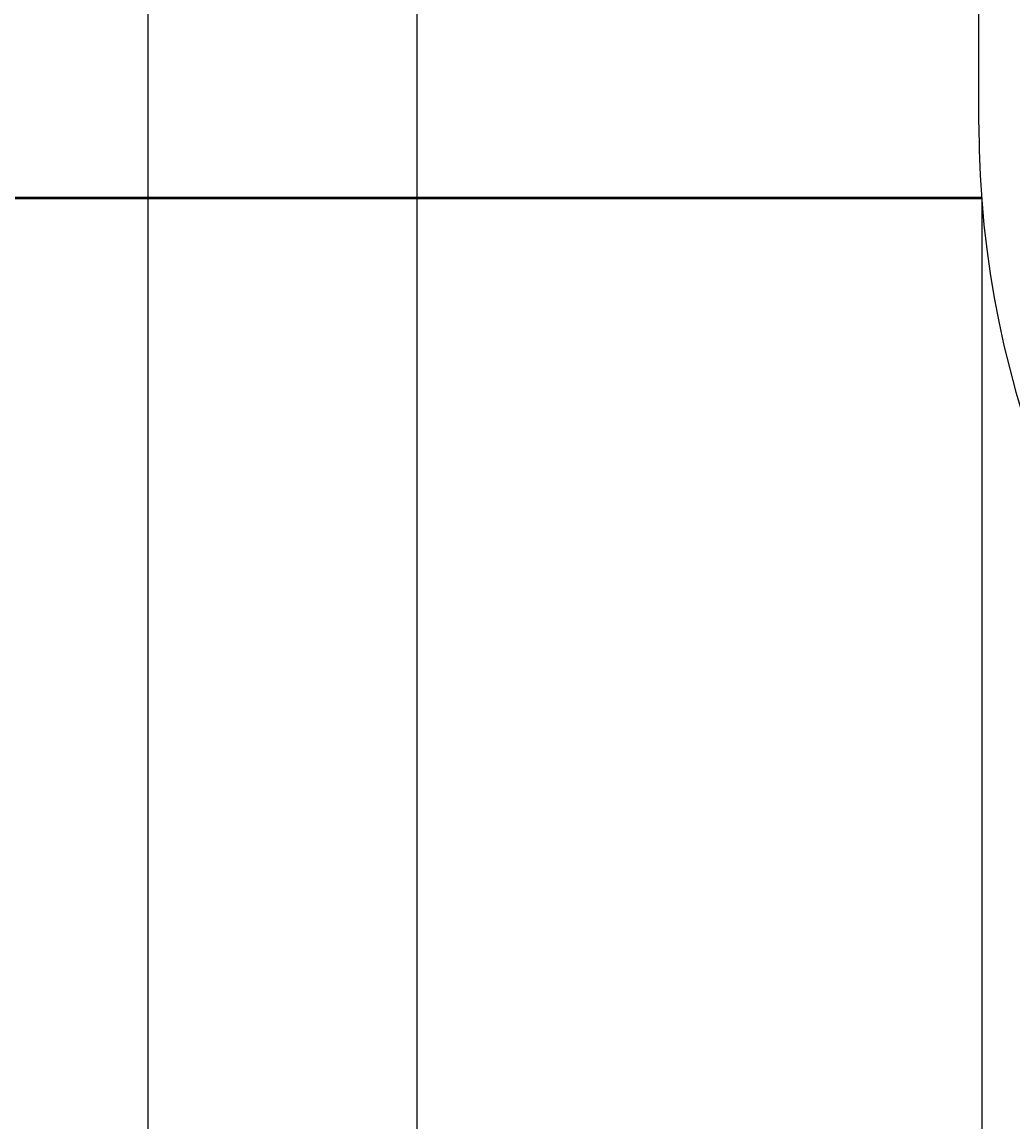
# Model space of a CAD drawing. Units: inches. Extents: x 37 to 824, y -700 to 234.
# Tile 34 of 77: x 211 to 251, y -206 to -161. Entities that reach past the tile are written whole.
import ezdxf

# ---------------------------------------------------------------- set-up
doc = ezdxf.new("R2010")
doc.units = ezdxf.units.IN
doc.header["$MEASUREMENT"] = 0
for name, color, linetype, lineweight in [('A-ANNO-DIMS', 2, 'Continuous', 18), ('A-DOOR', 4, 'Continuous', 25), ('A-WALL', 2, 'Continuous', 50)]:
    doc.layers.add(name, color=color, linetype=linetype, lineweight=lineweight)
doc.styles.get("Standard").update_dxf_attribs({"font": 'arial.ttf'})
doc.dimstyles.get("Standard").update_dxf_attribs({"dimtxt": 0.18, "dimasz": 0.18, "dimexe": 0.18, "dimexo": 0.0625, "dimgap": 0.09, "dimtad": 0, "dimtih": 1, "dimtoh": 1, "dimdec": 1, "dimzin": 0, "dimdsep": 46, "dimlunit": 4, "dimtxsty": 'Standard', "dimcen": 0.09, "dimadec": 0, "dimazin": 0, "dimtfac": 1, "dimtdec": 1, "dimtofl": 0, "dimtmove": 0, "dimatfit": 3, "dimfxl": 1, "dimtolj": 1, "dimtzin": 0, "dimarcsym": 0})

# ---------------------------------------------------------------- blocks, each defined once
blk = doc.blocks.new('*U2')
blk.add_line((-40, 0), (-40, 6))
blk.add_arc((0, 0), 40, 180, 270)
blk = doc.blocks.new('*D77')
at = {"layer": 'A-ANNO-DIMS', "color": 0, "lineweight": -2, "ltscale": 0.5, "transparency": 16777216}
for p, q in [((227.077, 45.5), (227.077, -400.406)), ((290.077, 15.028), (290.077, -400.406)), ((227.257, -400.226), (258.248, -400.226)), ((289.897, -400.226), (258.906, -400.226))]:
    blk.add_line(p, q, dxfattribs=at)
at = {"layer": 'A-ANNO-DIMS', "color": 0, "ltscale": 0.5, "transparency": 16777216}
for points in [[(227.257, -400.196), (227.257, -400.256), (227.077, -400.226)], [(289.897, -400.196), (289.897, -400.256), (290.077, -400.226)]]:
    blk.add_solid(points, dxfattribs=at)
at = {"layer": 'Defpoints', "color": 0, "ltscale": 0.5, "transparency": 16777216}
for p in [(227.077, 45.563), (290.077, 15.09), (290.077, -400.226)]:
    blk.add_point(p, dxfattribs=at)
at = {"layer": 'A-ANNO-DIMS', "color": 0, "ltscale": 0.5, "transparency": 16777216, "insert": (258.577, -400.226), "char_height": 0.18, "attachment_point": 5}
blk.add_mtext('\\A1;5\'-3"', dxfattribs=at)
blk = doc.blocks.new('*D80')
at = {"layer": 'A-ANNO-DIMS', "color": 0, "lineweight": -2, "ltscale": 0.5, "transparency": 16777216}
for p, q in [((170.077, -167.972), (170.077, -400.406)), ((250.19, -167.972), (250.19, -400.406)), ((170.257, -400.226), (209.804, -400.226)), ((250.01, -400.226), (210.463, -400.226))]:
    blk.add_line(p, q, dxfattribs=at)
at = {"layer": 'A-ANNO-DIMS', "color": 0, "ltscale": 0.5, "transparency": 16777216}
for points in [[(170.257, -400.196), (170.257, -400.256), (170.077, -400.226)], [(250.01, -400.196), (250.01, -400.256), (250.19, -400.226)]]:
    blk.add_solid(points, dxfattribs=at)
at = {"layer": 'Defpoints', "color": 0, "ltscale": 0.5, "transparency": 16777216}
for p in [(170.077, -167.91), (250.19, -167.91), (250.19, -400.226)]:
    blk.add_point(p, dxfattribs=at)
at = {"layer": 'A-ANNO-DIMS', "color": 0, "ltscale": 0.5, "transparency": 16777216, "insert": (210.133, -400.226), "char_height": 0.18, "attachment_point": 5}
blk.add_mtext('\\A1;6\'-8"', dxfattribs=at)
blk = doc.blocks.new('*D81')
at = {"layer": 'A-ANNO-DIMS', "color": 0, "lineweight": -2, "ltscale": 0.5, "transparency": 16777216}
for p, q in [((290.077, -164.972), (290.077, -400.406)), ((250.19, -167.972), (250.19, -400.406)), ((250.37, -400.226), (269.804, -400.226)), ((289.897, -400.226), (270.463, -400.226))]:
    blk.add_line(p, q, dxfattribs=at)
at = {"layer": 'A-ANNO-DIMS', "color": 0, "ltscale": 0.5, "transparency": 16777216}
for points in [[(250.37, -400.196), (250.37, -400.256), (250.19, -400.226)], [(289.897, -400.196), (289.897, -400.256), (290.077, -400.226)]]:
    blk.add_solid(points, dxfattribs=at)
at = {"layer": 'Defpoints', "color": 0, "ltscale": 0.5, "transparency": 16777216}
for p in [(290.077, -164.91), (250.19, -167.91), (290.077, -400.226)]:
    blk.add_point(p, dxfattribs=at)
at = {"layer": 'A-ANNO-DIMS', "color": 0, "ltscale": 0.5, "transparency": 16777216, "insert": (270.133, -400.226), "char_height": 0.18, "attachment_point": 5}
blk.add_mtext('\\A1;3\'-4"', dxfattribs=at)
blk = doc.blocks.new('*D86')
at = {"layer": 'A-ANNO-DIMS', "color": 0, "lineweight": -2, "ltscale": 0.5, "transparency": 16777216}
for p, q in [((206.077, -356.847), (206.077, 234.17)), ((206.257, 233.99), (210.678, 233.99)), ((215.897, 233.99), (211.476, 233.99)), ((216.077, -356.847), (216.077, 234.17))]:
    blk.add_line(p, q, dxfattribs=at)
at = {"layer": 'A-ANNO-DIMS', "color": 0, "ltscale": 0.5, "transparency": 16777216}
for points in [[(206.257, 234.02), (206.257, 233.96), (206.077, 233.99)], [(215.897, 234.02), (215.897, 233.96), (216.077, 233.99)]]:
    blk.add_solid(points, dxfattribs=at)
at = {"layer": 'Defpoints', "color": 0, "ltscale": 0.5, "transparency": 16777216}
for p in [(216.077, 233.99), (206.077, -356.91), (216.077, -356.91)]:
    blk.add_point(p, dxfattribs=at)
at = {"layer": 'A-ANNO-DIMS', "color": 0, "ltscale": 0.5, "transparency": 16777216, "insert": (211.077, 233.99), "char_height": 0.18, "attachment_point": 5}
blk.add_mtext('\\A1;0\'-10"', dxfattribs=at)
blk = doc.blocks.new('*D87')
at = {"layer": 'A-ANNO-DIMS', "color": 0, "lineweight": -2, "ltscale": 0.5, "transparency": 16777216}
for p, q in [((216.077, -356.847), (216.077, 234.17)), ((216.257, 233.99), (255.747, 233.99)), ((295.897, 233.99), (256.407, 233.99)), ((296.077, -356.847), (296.077, 234.17))]:
    blk.add_line(p, q, dxfattribs=at)
at = {"layer": 'A-ANNO-DIMS', "color": 0, "ltscale": 0.5, "transparency": 16777216}
for points in [[(216.257, 234.02), (216.257, 233.96), (216.077, 233.99)], [(295.897, 234.02), (295.897, 233.96), (296.077, 233.99)]]:
    blk.add_solid(points, dxfattribs=at)
at = {"layer": 'Defpoints', "color": 0, "ltscale": 0.5, "transparency": 16777216}
for p in [(296.077, 233.99), (216.077, -356.91), (296.077, -356.91)]:
    blk.add_point(p, dxfattribs=at)
at = {"layer": 'A-ANNO-DIMS', "color": 0, "ltscale": 0.5, "transparency": 16777216, "insert": (256.077, 233.99), "char_height": 0.18, "attachment_point": 5}
blk.add_mtext('\\A1;6\'-8"', dxfattribs=at)

msp = doc.modelspace()

# ---------------------------------------------------------------- linework, layer by layer
at = {"layer": 'A-WALL'}
msp.add_line((250.19, -167.91), (170.077, -167.91), dxfattribs=at)

# ---------------------------------------------------------------- block references
at = {"layer": 'A-DOOR'}
msp.add_blockref('*U2', (290.077, -164.91), dxfattribs=at)

# ---------------------------------------------------------------- dimensions: what is measured, and where the dimension line sits
at = {"layer": 'A-ANNO-DIMS', "ltscale": 0.5}
for base, p1, p2, picture, middle in [((216.077, 233.99), (206.077, -356.91), (216.077, -356.91), '*D86', (211.077, 233.99)), ((296.077, 233.99), (216.077, -356.91), (296.077, -356.91), '*D87', (256.077, 233.99)), ((290.077, -400.226), (227.077, 45.563), (290.077, 15.09), '*D77', (258.577, -400.226)), ((290.077, -400.226), (250.19, -167.91), (290.077, -164.91), '*D81', (270.133, -400.226)), ((250.19, -400.226), (170.077, -167.91), (250.19, -167.91), '*D80', (210.133, -400.226))]:
    dim = msp.add_linear_dim(base=base, p1=p1, p2=p2, dimstyle='Standard', override={"dimdec": 1, "dimlfac": 1, "dimrnd": 0, "dimzin": 1, "dimdsep": 46, "dimlunit": 4, "dimfrac": 2}, dxfattribs=at)
    dim.commit()
    dim.dimension.update_dxf_attribs({"geometry": picture, "text_midpoint": middle})

doc.saveas('drawing.dxf')
